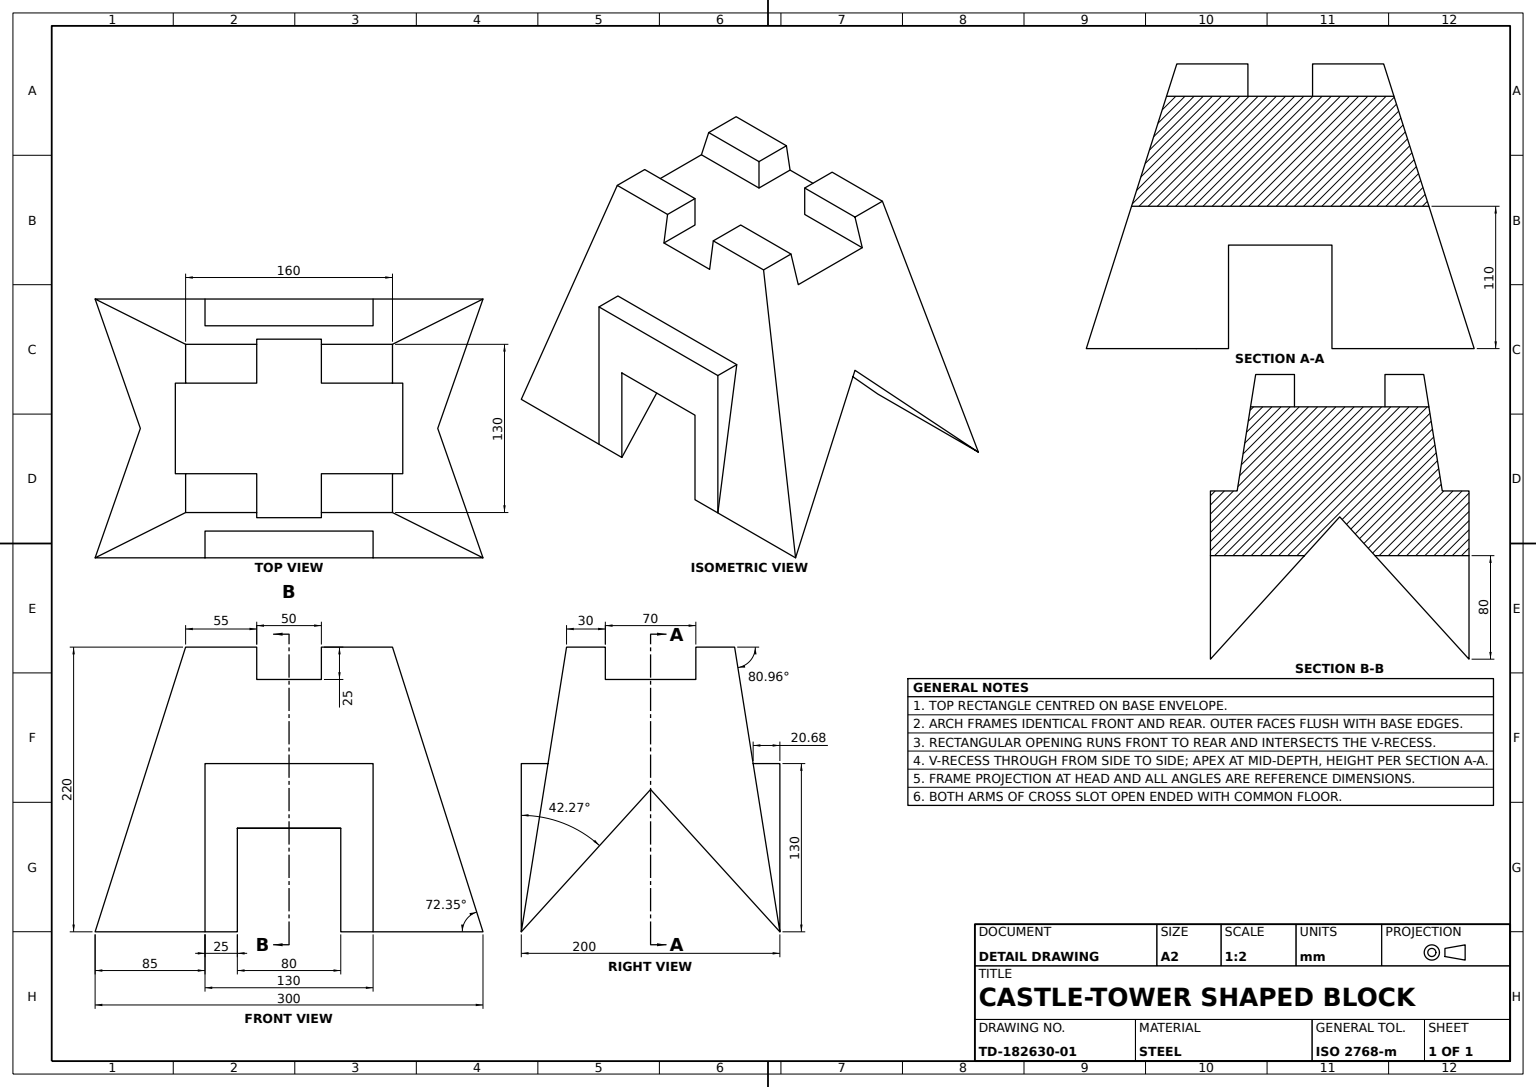
SolidWorks part; units mm, degrees
material "Plain Carbon Steel"
ref_plane "Front Plane" through (0, 0, 0) normal (0, 0, 1) x (1, 0, 0)
ref_plane "Top Plane" through (0, 0, 0) normal (0, 1, 0) x (1, 0, 0)
ref_plane "Right Plane" through (0, 0, 0) normal (1, 0, 0) x (0, 0, -1)
sketch "Base Profile Sketch" plane through (0, 0, 0) normal (1, 0, 0) x (0, 0, -1)
  line L0 (-150, 0) -> (-80, 220)
  line L1 (-80, 220) -> (-25, 220)
  line L2 (80, 220) -> (150, 0)
  line L3 (150, 0) -> (-150, 0)
  line L4 (0, 0) -> (0, 220) construction
  line L5 (25, 220) -> (80, 220)
  line L7 (-25, 220) -> (-25, 195)
  line L8 (-25, 195) -> (25, 195)
  line L9 (25, 220) -> (25, 195)
  dimension "D1" = 220
  dimension "D2" = 300
  dimension "D3" = 160
  dimension "D4" = 55
  dimension "D5" = 25
extrude "Inclined Base Block" add sketch "Base Profile Sketch" along normal mid plane 200
sketch "Front Notch Sketch" plane through (0, 0, 0) normal (0, 0, 1) x (1, 0, 0)
  line L0 (-100, 0) -> (-65, 220)
  line L1 (100, 220) -> (-100, 220) construction
  line L2 (-65, 220) -> (-35, 220)
  line L3 (65, 220) -> (100, 0)
  line L4 (100, 0) -> (-100, 0)
  line L5 (0, 220) -> (0, 0) construction
  line L6 (35, 220) -> (65, 220)
  line L8 (-35, 220) -> (-35, 195)
  line L9 (-35, 195) -> (35, 195)
  line L10 (35, 220) -> (35, 195)
  dimension "D1" = 130
  dimension "D2" = 30
  dimension "D3" = 25
extrude "Front Notch Cut" cut sketch "Front Notch Sketch" against normal through all both and the other way through all flip side to cut
sketch "Top Recess Sketch" plane through (0, 0, 0) normal (0, 0, 1) x (1, 0, 0)
  line L0 (-100, 0) -> (0, 110)
  line L1 (0, 110) -> (100, 0)
  line L2 (100, 0) -> (-100, 0) construction
  line L3 (0, 0) -> (0, 110) construction
  line L4 (-100, 0) -> (100, 0)
  dimension "D1" = 110
extrude "Top Recess Cut" cut sketch "Top Recess Sketch" against normal through all both and the other way through all
sketch "Front Frame Sketch" plane through (0, 0, 0) normal (0, 0, 1) x (1, 0, 0)
  line L0 (100, 0) -> (100, 130)
  line L1 (100, 130) -> (79.3182, 130)
  line L2 (65, 220) -> (100, 0) construction
  line L3 (79.3182, 130) -> (100, 0)
  dimension "D1" = 130
extrude "Front Frame Boss" add sketch "Front Frame Sketch" along normal mid plane 130
mirror "Front Frame Mirror" about plane through (0, 0, 0) normal (1, 0, 0) of "Front Frame Boss"
sketch "Top Cross Slot Sketch" plane through (100, 0, 0) normal (1, 0, 0) x (0, 0, -1)
  line L0 (-65, 0) -> (65, 0) construction
  line L1 (-40, 0) -> (40, 0)
  line L2 (-40, 0) -> (-40, 80)
  line L3 (-40, 80) -> (40, 80)
  line L4 (40, 0) -> (40, 80)
  line L5 (0, 0) -> (0, 80) construction
  dimension "D1" = 80
  dimension "D2" = 80
extrude "Top Cross Slot Cut 80x80" cut sketch "Top Cross Slot Sketch" against normal through all both and the other way through all
